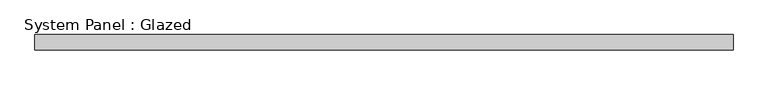
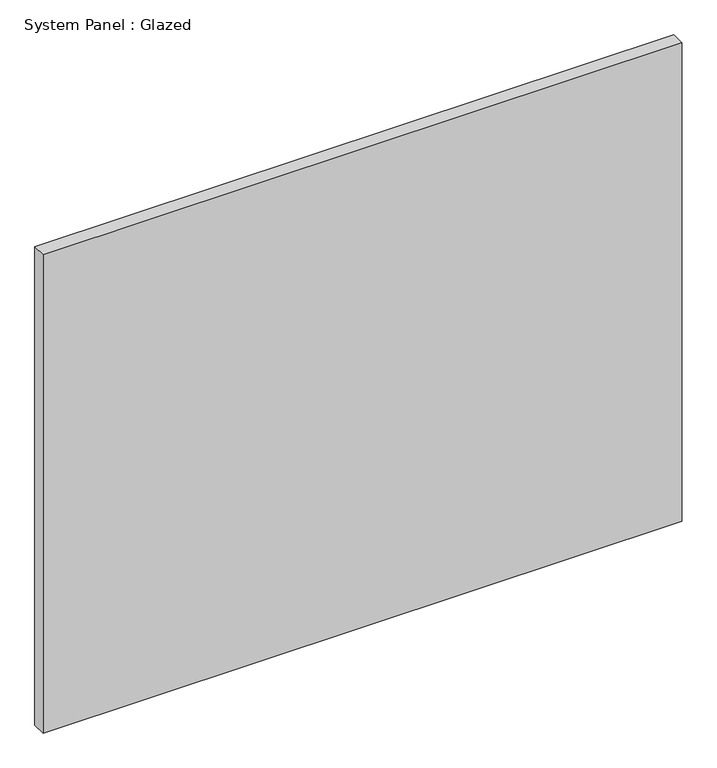
"""IFC4 building model written with IfcOpenShell, lengths in millimetres: plate geometry, System Panel : Glazed."""

from ifc_helpers import new_model, si_unit, origin, origin_with_axes, place, context, project, spatial, polyline, outline, extrude, source, transform, mapped, element, save


def system_panel_glazed_2060cbb7(model_context):
    return source(origin(), model_context, "Body", "SweptSolid", [
        extrude(outline(polyline([(577.9180043, 19.05), (-577.9180043, 19.05), (-577.9180043, 44.45), (577.9180043, 44.45), (577.9180043, 19.05)])), origin_with_axes(), (0.0, 0.0, 1.0), 914.4),
    ])


if __name__ == "__main__":
    model = new_model("IFC4")
    model_context = context("Model", 3, world=origin())
    ifc_project = project(units=[si_unit("LENGTHUNIT", "METRE", prefix="MILLI")], contexts=[model_context])
    site = spatial("IfcSite", under=ifc_project)
    building = spatial("IfcBuilding", under=site)
    placement = place(None, origin())
    system_panel_glazed_shape = system_panel_glazed_2060cbb7(model_context)
    element("IfcPlate", 1, ObjectType="System Panel : Glazed", at=placement, inside=building, context=model_context, shape_type="MappedRepresentation", body=[
        mapped(system_panel_glazed_shape, transform((0.0, 0.0, 0.0), x_axis=(1.0, 0.0, 0.0), y_axis=(0.0, 1.0, 0.0), z_axis=(0.0, 0.0, 1.0))),
    ])
    save(model, "model.ifc")

# Revit data of these elements
# Type "System Panel : Glazed"
#   Construction Type Id = "GSP4R"
#   Analytic Construction = "1/8 in Pilkington single glazing"
#   Visual Light Transmittance = 0.9
#   Solar Heat Gain Coefficient = 0.86
#   Heat Transfer Coefficient (U) = 1.18115 BTU/(h·ft²·°F)
# Element 1 (IfcPlate, "System Panel : Glazed")
#   Materials on its faces: "Glass"
# Materials
#   "Glass": class "Glass", colour RGB 0 128 192, transparency 0.75, Description = "Soda Lime Glass", Cost = 0
